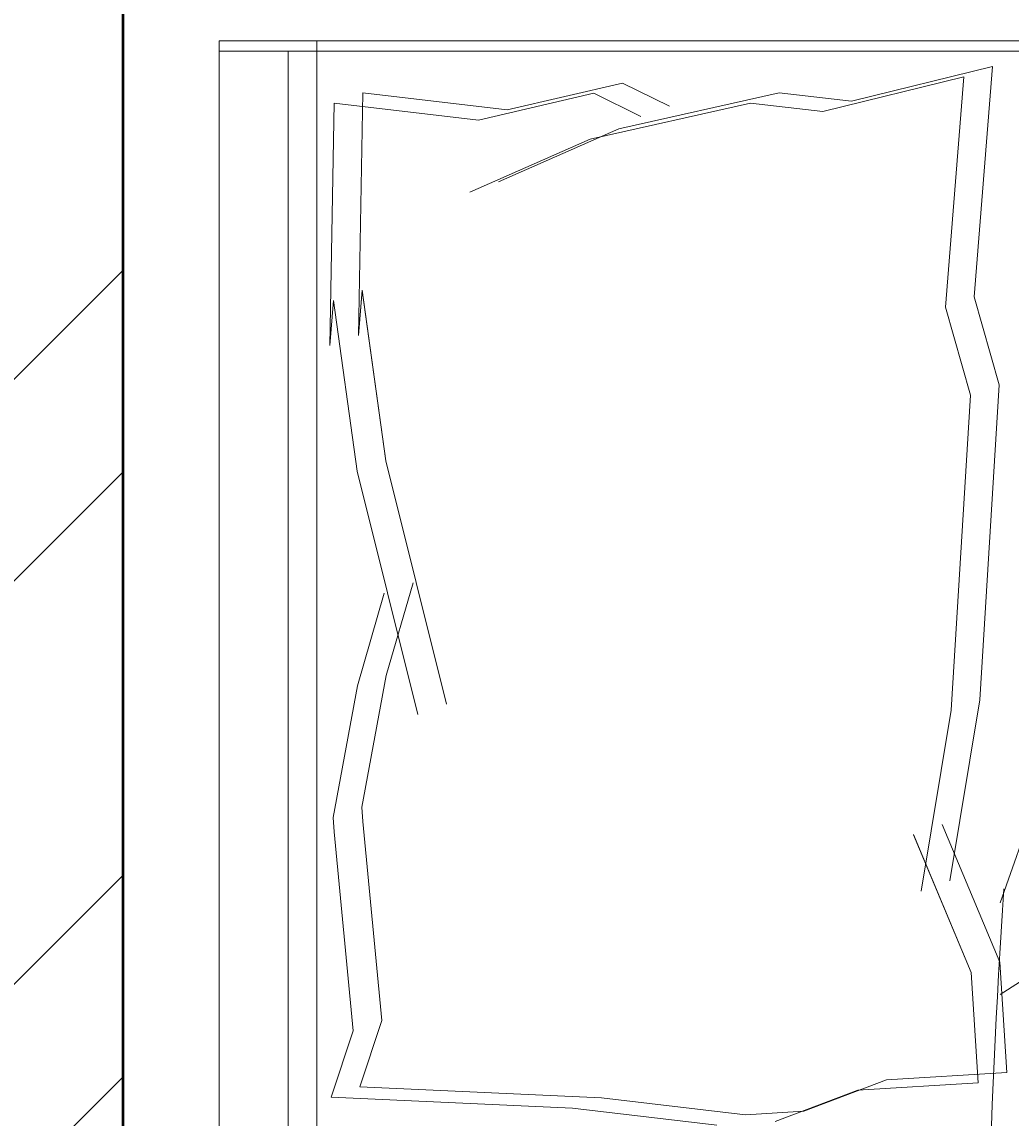
# Model space of a CAD drawing. Units: inches. Extents: x 963 to 2075, y 289 to 2657.
# Tile 39 of 98: x 1511 to 1533, y 1615 to 1640. Entities that reach past the tile are written whole.
import ezdxf

# ---------------------------------------------------------------- set-up
doc = ezdxf.new("R2010")
doc.units = ezdxf.units.IN
for name, color, linetype, lineweight in [('A-ANNO-DIMS', 2, 'Continuous', 18), ('A-FURN', 8, 'Continuous', 18), ('A-WALL', 7, 'Continuous', 50), ('A-WALL-PATT', 8, 'Continuous', 13)]:
    doc.layers.add(name, color=color, linetype=linetype, lineweight=lineweight)
doc.styles.get("Standard").update_dxf_attribs({"font": 'arial.ttf'})
doc.dimstyles.get("Standard").update_dxf_attribs({"dimtxt": 0.18, "dimasz": 0.18, "dimexe": 0.18, "dimexo": 0.0625, "dimgap": 0.09, "dimtad": 0, "dimtih": 1, "dimtoh": 1, "dimdec": 4, "dimzin": 0, "dimdsep": 46, "dimtxsty": 'Standard', "dimcen": 0.09, "dimadec": 0, "dimazin": 0, "dimtfac": 1, "dimtdec": 4, "dimtofl": 0, "dimtmove": 0, "dimatfit": 3, "dimfxl": 1, "dimtolj": 1, "dimtzin": 0, "dimarcsym": 0})

# ---------------------------------------------------------------- blocks, each defined once
blk = doc.blocks.new('BED-DOUBLE')
for p, q in [((1252.699, 2450.52), (1252.699, 2402.729)), ((1252.699, 2450.519), (1252.699, 2402.729)), ((1253.338, 2450.748), (1253.338, 2402.958)), ((1253.338, 2450.748), (1253.338, 2402.958)), ((1254.872, 2450.748), (1254.872, 2402.729)), ((1247.005, 2426.489), (1243.794, 2426.868)), ((1247.005, 2426.49), (1243.794, 2426.868)), ((1242.495, 2426.787), (1240.655, 2426.093)), ((1242.495, 2426.787), (1240.655, 2426.093)), ((1243.154, 2426.64), (1241.856, 2426.559)), ((1243.154, 2426.64), (1241.856, 2426.559)), ((1246.365, 2426.261), (1243.154, 2426.64)), ((1246.365, 2426.261), (1243.154, 2426.64)), ((1241.856, 2426.559), (1240.016, 2425.864)), ((1241.856, 2426.559), (1240.016, 2425.865)), ((1252.38, 2426.246), (1247.005, 2426.49)), ((1252.38, 2426.246), (1247.005, 2426.489)), ((1251.741, 2426.018), (1246.365, 2426.261)), ((1251.741, 2426.018), (1246.365, 2426.261)), ((1251.893, 2424.767), (1252.38, 2426.246)), ((1251.893, 2424.768), (1252.38, 2426.246)), ((1240.016, 2425.865), (1237.34, 2425.697)), ((1240.016, 2425.864), (1237.34, 2425.697)), ((1240.655, 2426.093), (1237.979, 2425.925)), ((1240.655, 2426.093), (1237.979, 2425.926)), ((1237.979, 2425.926), (1238.132, 2423.473)), ((1237.979, 2425.925), (1238.132, 2423.473)), ((1251.254, 2424.539), (1251.741, 2426.018)), ((1251.254, 2424.539), (1251.741, 2426.018)), ((1237.34, 2425.697), (1237.493, 2423.244)), ((1237.34, 2425.697), (1237.493, 2423.245)), ((1252.315, 2420.34), (1251.893, 2424.768)), ((1252.315, 2420.339), (1251.893, 2424.767)), ((1251.675, 2420.111), (1251.254, 2424.539)), ((1251.675, 2420.111), (1251.254, 2424.539)), ((1237.488, 2423.964), (1230.995, 2419.774)), ((1237.488, 2423.964), (1230.995, 2419.774)), ((1238.132, 2423.473), (1239.417, 2420.402)), ((1238.132, 2423.473), (1239.417, 2420.403)), ((1237.493, 2423.245), (1238.778, 2420.174)), ((1237.493, 2423.244), (1238.778, 2420.174)), ((1234.555, 2413.579), (1237.488, 2421.917)), ((1234.555, 2413.579), (1237.488, 2421.917)), ((1239.243, 2421.659), (1238.577, 2417.627)), ((1239.243, 2421.659), (1238.577, 2417.627)), ((1238.604, 2421.431), (1237.937, 2417.399)), ((1238.604, 2421.43), (1237.937, 2417.398)), ((1252.335, 2420.019), (1252.315, 2420.34)), ((1252.335, 2420.018), (1252.315, 2420.339)), ((1251.695, 2419.79), (1251.675, 2420.111)), ((1251.695, 2419.79), (1251.675, 2420.111)), ((1251.793, 2417.088), (1252.335, 2420.019)), ((1251.793, 2417.088), (1252.335, 2420.018)), ((1251.154, 2416.859), (1251.695, 2419.79)), ((1251.154, 2416.86), (1251.695, 2419.79)), ((1238.577, 2417.627), (1238.145, 2410.617)), ((1238.577, 2417.627), (1238.145, 2410.617)), ((1251.802, 2412.309), (1250.45, 2417.728)), ((1251.802, 2412.309), (1250.45, 2417.728)), ((1237.937, 2417.399), (1237.506, 2410.389)), ((1237.937, 2417.398), (1237.506, 2410.388)), ((1251.163, 2412.08), (1249.81, 2417.5)), ((1251.163, 2412.081), (1249.81, 2417.5)), ((1251.198, 2415.023), (1251.793, 2417.088)), ((1251.198, 2415.023), (1251.793, 2417.088)), ((1250.559, 2414.795), (1251.154, 2416.86)), ((1250.559, 2414.794), (1251.154, 2416.859)), ((1252.329, 2408.511), (1251.802, 2412.309)), ((1252.329, 2408.511), (1251.802, 2412.309)), ((1251.69, 2408.283), (1251.163, 2412.081)), ((1251.69, 2408.282), (1251.163, 2412.08)), ((1238.145, 2410.617), (1238.703, 2408.656)), ((1238.145, 2410.617), (1238.703, 2408.657)), ((1237.506, 2410.389), (1238.063, 2408.428)), ((1237.506, 2410.388), (1238.063, 2408.428)), ((1252.315, 2404.111), (1252.412, 2409.514)), ((1252.315, 2404.111), (1252.412, 2409.513)), ((1252.412, 2409.514), (1252.329, 2408.511)), ((1252.412, 2409.513), (1252.329, 2408.511)), ((1251.675, 2403.883), (1251.772, 2409.285)), ((1251.675, 2403.883), (1251.772, 2409.285)), ((1251.772, 2409.285), (1251.69, 2408.282)), ((1251.772, 2409.285), (1251.69, 2408.283)), ((1238.703, 2408.657), (1238.299, 2403.525)), ((1238.703, 2408.656), (1238.299, 2403.525)), ((1238.063, 2408.428), (1237.66, 2403.296)), ((1238.063, 2408.428), (1237.66, 2403.297)), ((1246.615, 2404.913), (1249.293, 2406.095)), ((1246.615, 2404.914), (1249.293, 2406.095)), ((1245.975, 2404.685), (1248.654, 2405.867)), ((1245.975, 2404.685), (1248.654, 2405.866)), ((1243.043, 2404.111), (1246.615, 2404.914)), ((1243.043, 2404.111), (1246.615, 2404.913)), ((1242.404, 2403.882), (1245.975, 2404.685)), ((1242.404, 2403.883), (1245.975, 2404.685)), ((1246.533, 2403.895), (1245.487, 2404.409)), ((1246.533, 2403.894), (1245.487, 2404.408)), ((1249.104, 2404.49), (1246.533, 2403.894)), ((1249.104, 2404.49), (1246.533, 2403.895)), ((1252.315, 2404.111), (1249.104, 2404.49)), ((1252.315, 2404.111), (1249.104, 2404.49)), ((1238.299, 2403.525), (1241.438, 2404.3)), ((1238.299, 2403.525), (1241.438, 2404.3)), ((1241.438, 2404.3), (1243.043, 2404.111)), ((1241.438, 2404.3), (1243.043, 2404.111)), ((1245.894, 2403.666), (1244.848, 2404.18)), ((1245.894, 2403.666), (1244.848, 2404.18)), ((1248.465, 2404.262), (1245.894, 2403.666)), ((1248.465, 2404.261), (1245.894, 2403.666)), ((1251.675, 2403.883), (1248.465, 2404.262)), ((1251.675, 2403.883), (1248.465, 2404.261)), ((1237.66, 2403.296), (1240.798, 2404.072)), ((1237.66, 2403.297), (1240.798, 2404.072)), ((1240.798, 2404.072), (1242.404, 2403.882)), ((1240.798, 2404.072), (1242.404, 2403.883)), ((1254.872, 2402.958), (1228.262, 2402.958)), ((1254.872, 2402.958), (1228.262, 2402.958)), ((1254.232, 2402.729), (1227.623, 2402.729)), ((1254.232, 2402.729), (1227.623, 2402.729)), ((1254.872, 2402.729), (1254.232, 2402.729))]:
    blk.add_line(p, q)
blk.add_arc((1072.819, 2432.864), 164.969, 356.08655, 6.78213)
blk.add_arc((1072.819, 2432.864), 164.969, 356.08655, 6.78213)
blk = doc.blocks.new('*D15')
at = {"layer": 'A-ANNO-DIMS', "color": 0, "lineweight": -2, "transparency": 16777216}
for p, q in [((1515.003, 1643.505), (1502.653, 1643.505)), ((1502.833, 1643.325), (1502.833, 1615.775)), ((1502.833, 1587.861), (1502.833, 1615.411)), ((1515.003, 1587.681), (1502.653, 1587.681))]:
    blk.add_line(p, q, dxfattribs=at)
at = {"layer": 'A-ANNO-DIMS', "color": 0, "transparency": 16777216}
for points in [[(1502.803, 1643.325), (1502.863, 1643.325), (1502.833, 1643.505)], [(1502.803, 1587.861), (1502.863, 1587.861), (1502.833, 1587.681)]]:
    blk.add_solid(points, dxfattribs=at)
at = {"layer": 'Defpoints', "color": 0, "transparency": 16777216}
for p in [(1515.065, 1643.505), (1502.833, 1587.681), (1515.065, 1587.681)]:
    blk.add_point(p, dxfattribs=at)
at = {"layer": 'A-ANNO-DIMS', "color": 0, "transparency": 16777216, "insert": (1502.833, 1615.593), "char_height": 0.18, "attachment_point": 5}
blk.add_mtext('\\A1;56 TYP.', dxfattribs=at)

msp = doc.modelspace()

# ---------------------------------------------------------------- hatches: boundary and pattern name
at = {"layer": 'A-WALL-PATT'}
h = msp.add_hatch(dxfattribs=at)
h.set_pattern_fill('ANSI32', color=256)
h.paths.add_polyline_path([(1473.609, 2163.068), (1473.609, 2165.318), (1376.422, 2165.318), (1376.422, 2227.983), (1371.922, 2227.983), (1371.922, 2214.818), (1368.405, 2214.818), (1368.405, 2210.318), (1371.922, 2210.318), (1371.922, 2160.818), (1395.922, 2160.818), (1395.922, 2090.318), (1217.345, 2090.318), (1217.345, 2085.818), (1395.922, 2085.818), (1458.922, 2085.818), (1458.922, 2108.318), (1454.422, 2108.318), (1454.422, 2090.318), (1400.422, 2090.318), (1400.422, 2160.818), (1473.609, 2160.818)])
h.paths.add_polyline_path([(1649.422, 2210.318), (1653.225, 2210.318), (1653.225, 2214.818), (1649.422, 2214.818), (1649.422, 2227.983), (1644.922, 2227.983), (1644.922, 2165.318), (1550.099, 2165.318), (1550.099, 2160.818), (1620.922, 2160.818), (1620.922, 2112.818), (1555.446, 2112.818), (1555.446, 2108.318), (1584.327, 2108.318), (1584.327, 2084.916), (1588.827, 2084.916), (1588.827, 2108.318), (1625.422, 2108.318), (1667.951, 2108.318), (1667.951, 2022.667), (1588.827, 2022.667), (1588.827, 2047.408), (1584.327, 2047.408), (1584.327, 1996.003), (1588.827, 1996.003), (1588.827, 2018.318), (1667.951, 2018.167), (1667.951, 1928.318), (1625.422, 1928.318), (1625.422, 1923.818), (1672.451, 1923.818), (1672.451, 1928.318), (1672.451, 1946.663), (1785.446, 1946.663), (1785.446, 1951.163), (1743.034, 1951.163), (1743.034, 2017.922), (1841.422, 2017.922), (1841.422, 2014.775), (1845.922, 2014.775), (1845.922, 2017.922), (1905.922, 2017.922), (1905.922, 1987.511), (1910.422, 1987.511), (1910.422, 2022.422), (1910.422, 2068.517), (1905.922, 2068.517), (1905.922, 2022.422), (1845.922, 2022.422), (1845.922, 2025.851), (1843.672, 2025.851), (1841.422, 2025.851), (1841.422, 2022.422), (1743.034, 2022.422), (1743.034, 2084.031), (1768.451, 2084.031), (1785.446, 2084.031), (1785.446, 2088.531), (1672.451, 2088.531), (1672.451, 2112.818), (1667.951, 2112.818), (1625.422, 2112.818), (1625.422, 2160.818), (1649.422, 2160.818)])
h.paths.add_polyline_path([(1672.451, 2084.031), (1738.534, 2084.031), (1738.534, 1951.163), (1672.451, 1951.163)], flags=16)
h.paths.add_polyline_path([(1672.451, 2084.031), (1738.534, 2084.031), (1705.492, 2017.597)], flags=0)
h.paths.add_polyline_path([(1262.766, 2085.818), (1258.266, 2085.818), (1258.266, 2023.278), (1184.422, 2023.278), (1184.422, 2018.778), (1258.266, 2018.778), (1258.266, 1950.818), (1262.766, 1950.818)])
h.paths.add_polyline_path([(1312.266, 2085.818), (1307.766, 2085.818), (1307.766, 1950.818), (1312.266, 1950.818)])
h.paths.add_polyline_path([(1458.922, 1950.818), (1395.922, 1950.818), (1216.568, 1950.818), (1216.568, 1946.318), (1346.422, 1946.318), (1395.922, 1946.318), (1395.922, 1875.818), (1371.922, 1875.818), (1371.922, 1826.318), (1368.931, 1826.318), (1368.931, 1821.818), (1371.922, 1821.818), (1371.922, 1813.622), (1376.422, 1813.622), (1376.422, 1871.318), (1474.504, 1871.318), (1474.504, 1873.568), (1474.504, 1875.818), (1400.422, 1875.818), (1400.422, 1946.318), (1454.422, 1946.318), (1454.422, 1928.318), (1458.922, 1928.318)])
h.paths.add_polyline_path([(1184.422, 2120.778), (1167.922, 2120.778), (1167.922, 2134.812), (1165.672, 2134.812), (1163.422, 2134.812), (1163.422, 2120.778), (1119.922, 2120.778), (1119.922, 2098.095), (1124.422, 2098.095), (1124.422, 2116.278), (1167.922, 2116.278), (1179.922, 2116.278), (1179.922, 2045.916), (1184.422, 2045.916), (1184.422, 2090.318), (1184.422, 2116.278)])
h.paths.add_polyline_path([(1124.422, 2018.778), (1179.922, 2018.778), (1179.922, 2016.294), (1184.422, 2016.294), (1184.422, 2023.278), (1184.422, 2026.588), (1182.172, 2026.588), (1179.922, 2026.588), (1179.922, 2023.278), (1124.422, 2023.278), (1124.422, 2074.095), (1119.922, 2074.095), (1119.922, 2018.778), (1119.922, 1979.633), (1124.422, 1979.633)])
h.paths.add_polyline_path([(1184.422, 1925.778), (1184.422, 1946.318), (1184.422, 1996.073), (1182.172, 1996.073), (1179.922, 1996.073), (1179.922, 1925.778), (1124.422, 1925.778), (1124.422, 1955.633), (1119.922, 1955.502), (1119.922, 1921.278), (1158.922, 1921.278), (1158.922, 1909.983), (1163.422, 1909.983), (1163.422, 1921.278), (1184.422, 1921.278)])
h.paths.add_polyline_path([(1341.449, 1826.318), (1163.422, 1826.318), (1163.422, 1849.983), (1158.922, 1849.983), (1158.922, 1821.818), (1158.922, 1804.033), (1163.422, 1804.033), (1163.422, 1821.818), (1341.449, 1821.818)])
h.paths.add_polyline_path([(1222.981, 1713.818), (1163.422, 1713.818), (1163.422, 1744.033), (1161.172, 1744.033), (1158.922, 1744.033), (1158.922, 1713.818), (1119.922, 1713.818), (1119.922, 1694.65), (1124.422, 1694.65), (1124.422, 1709.318), (1158.922, 1709.318), (1222.981, 1709.318)])
h.paths.add_polyline_path([(1328.422, 1713.818), (1252.042, 1713.818), (1252.042, 1711.568), (1252.042, 1709.318), (1256.422, 1709.318), (1256.422, 1547.318), (1232.937, 1547.318), (1232.937, 1545.068), (1232.937, 1542.818), (1292.422, 1542.818), (1292.422, 1527.634), (1296.922, 1527.634), (1296.922, 1542.818), (1299.464, 1542.818), (1299.464, 1547.318), (1260.922, 1547.318), (1260.922, 1658.318), (1343.661, 1658.318), (1343.661, 1660.568), (1343.661, 1662.818), (1328.422, 1662.818), (1328.422, 1676.589), (1327.402, 1676.589), (1323.922, 1676.589), (1323.922, 1662.818), (1260.922, 1662.818), (1260.922, 1709.318), (1323.922, 1709.318), (1323.922, 1699.851), (1328.422, 1699.851)])
h.paths.add_polyline_path([(1649.422, 1875.818), (1625.422, 1875.818), (1625.422, 1928.318), (1620.922, 1928.318), (1588.827, 1928.318), (1588.827, 1950.59), (1584.327, 1950.59), (1584.327, 1928.318), (1555.446, 1928.318), (1555.446, 1923.818), (1620.922, 1923.818), (1620.922, 1875.818), (1548.952, 1875.818), (1548.952, 1873.568), (1548.952, 1871.318), (1644.922, 1871.318), (1644.922, 1813.622), (1649.422, 1813.622), (1649.422, 1821.818), (1652.045, 1821.818), (1652.045, 1824.068), (1652.045, 1826.318), (1649.422, 1826.318)])
h.paths.add_polyline_path([(1512.922, 1871.318), (1516.476, 1871.318), (1516.476, 1875.818), (1512.922, 1875.818), (1512.922, 1923.818), (1512.922, 1928.318), (1512.922, 1930.827), (1508.422, 1930.827), (1508.422, 1875.818), (1504.411, 1875.818), (1504.411, 1871.318), (1508.422, 1871.318), (1508.422, 1713.818), (1376.422, 1713.818), (1376.422, 1743.325), (1371.922, 1743.325), (1371.922, 1709.318), (1371.922, 1706.01), (1376.422, 1706.01), (1376.422, 1709.318), (1508.422, 1709.318), (1508.422, 1547.318), (1501.871, 1547.318), (1501.871, 1542.818), (1508.422, 1542.818), (1508.422, 1482.818), (1508.422, 1436.318), (1512.922, 1436.318), (1512.922, 1542.818), (1519.318, 1542.818), (1519.318, 1545.068), (1519.318, 1547.318), (1512.922, 1547.318), (1512.922, 1709.318), (1644.922, 1709.318), (1644.922, 1707.548), (1649.422, 1707.548), (1649.422, 1709.318), (1649.422, 1743.325), (1644.922, 1743.325), (1644.922, 1713.818), (1512.922, 1713.818)])
h.paths.add_polyline_path([(1129.884, 1545.068), (1129.884, 1547.318), (1124.422, 1547.318), (1095.922, 1547.318), (1095.922, 1614.818), (1124.422, 1614.818), (1124.422, 1619.318), (1095.922, 1619.318), (1091.422, 1619.318), (1091.422, 1542.818), (1095.922, 1542.818), (1119.922, 1542.818), (1129.884, 1542.818)])
h.paths.add_polyline_path([(1208.422, 1542.818), (1211.74, 1542.818), (1211.74, 1547.318), (1198.851, 1547.318), (1198.851, 1542.818), (1203.922, 1542.818), (1203.922, 1478.318), (1208.422, 1478.318), (1296.922, 1478.318), (1296.922, 1503.634), (1292.422, 1503.634), (1292.422, 1482.818), (1208.422, 1482.818)])
h.paths.add_polyline_path([(1430.422, 1542.818), (1435.699, 1542.818), (1435.699, 1545.068), (1435.699, 1547.318), (1422.658, 1547.318), (1422.658, 1545.068), (1422.658, 1542.818), (1425.922, 1542.818), (1425.922, 1482.857), (1341.922, 1482.857), (1341.922, 1502.732), (1337.422, 1502.732), (1337.422, 1478.357), (1425.922, 1478.357), (1425.922, 1440.818), (1425.922, 1436.318), (1430.422, 1436.318)])
h.paths.add_polyline_path([(1698.482, 2004.259), (1727.695, 2004.259), (1727.695, 2022.916), (1698.482, 2022.916)], flags=8)

# ---------------------------------------------------------------- linework, layer by layer
at = {"layer": 'A-WALL'}
msp.add_line((1512.922, 1547.318), (1512.922, 1709.318), dxfattribs=at)

# ---------------------------------------------------------------- block references
at = {"layer": 'A-FURN', "rotation": 180}
msp.add_blockref('BED-DOUBLE', (2769.937, 4041.99), dxfattribs=at)

# ---------------------------------------------------------------- dimensions: what is measured, and where the dimension line sits
at = {"layer": 'A-ANNO-DIMS'}
dim = msp.add_linear_dim(base=(1502.833, 1587.681), p1=(1515.065, 1643.505), p2=(1515.065, 1587.681), angle=270, text='<> TYP.', dimstyle='Standard', override={"dimdec": 0, "dimlfac": 1, "dimrnd": 0, "dimzin": 0, "dimdsep": 46, "dimlunit": 2}, dxfattribs=at)
dim.commit()
dim.dimension.update_dxf_attribs({"geometry": '*D15', "text_midpoint": (1502.833, 1615.593)})

doc.saveas('drawing.dxf')
